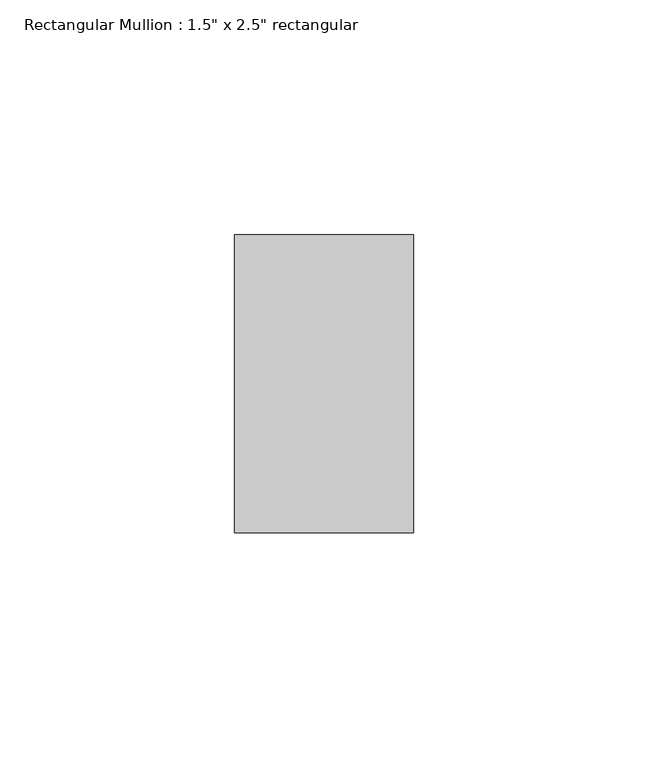
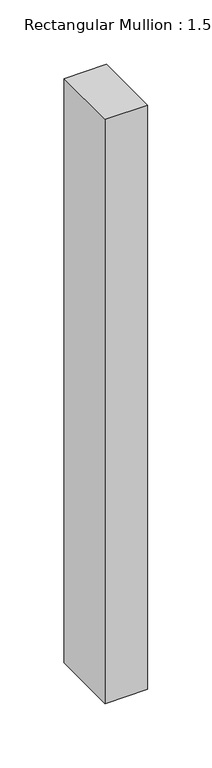
"""IFC4 building model written with IfcOpenShell, lengths in millimetres: member geometry."""

from ifc_helpers import new_model, si_unit, frame, origin, place, context, project, spatial, polyline, outline, extrude, source, transform, mapped, element, save


def member_bb410062(model_context):
    return source(origin(), model_context, "Body", "SweptSolid", [
        extrude(outline(polyline([(19.05, 31.75), (19.05, -31.75), (-19.05, -31.75), (-19.05, 31.75), (19.05, 31.75)])), frame((0.0, 0.0, -553.3665215), z_axis=(0.0, 0.0, 1.0), x_axis=(1.0, 0.0, 0.0)), (0.0, 0.0, 1.0), 553.3665215),
    ])


if __name__ == "__main__":
    model = new_model("IFC4")
    model_context = context("Model", 3, world=origin())
    ifc_project = project(units=[si_unit("LENGTHUNIT", "METRE", prefix="MILLI")], contexts=[model_context])
    site = spatial("IfcSite", under=ifc_project)
    building = spatial("IfcBuilding", under=site)
    placement = place(None, origin())
    member_shape = member_bb410062(model_context)
    element("IfcMember", 1, ObjectType="Rectangular Mullion : 1.5\" x 2.5\" rectangular", at=placement, inside=building, context=model_context, shape_type="MappedRepresentation", body=[
        mapped(member_shape, transform((0.0, 0.0, 0.0), x_axis=(1.0, 0.0, 0.0), y_axis=(0.0, 1.0, 0.0), z_axis=(0.0, 0.0, 1.0))),
    ])
    save(model, "model.ifc")

# Revit data of these elements
# Type "Rectangular Mullion : 1.5\" x 2.5\" rectangular"
#   built-in parameter 1007304 = 0.208333 (stored number, unit not read)
#   built-in parameter 1007301 = 0.0625 (stored number, unit not read)
#   built-in parameter 1007300 = 0.0625 (stored number, unit not read)
